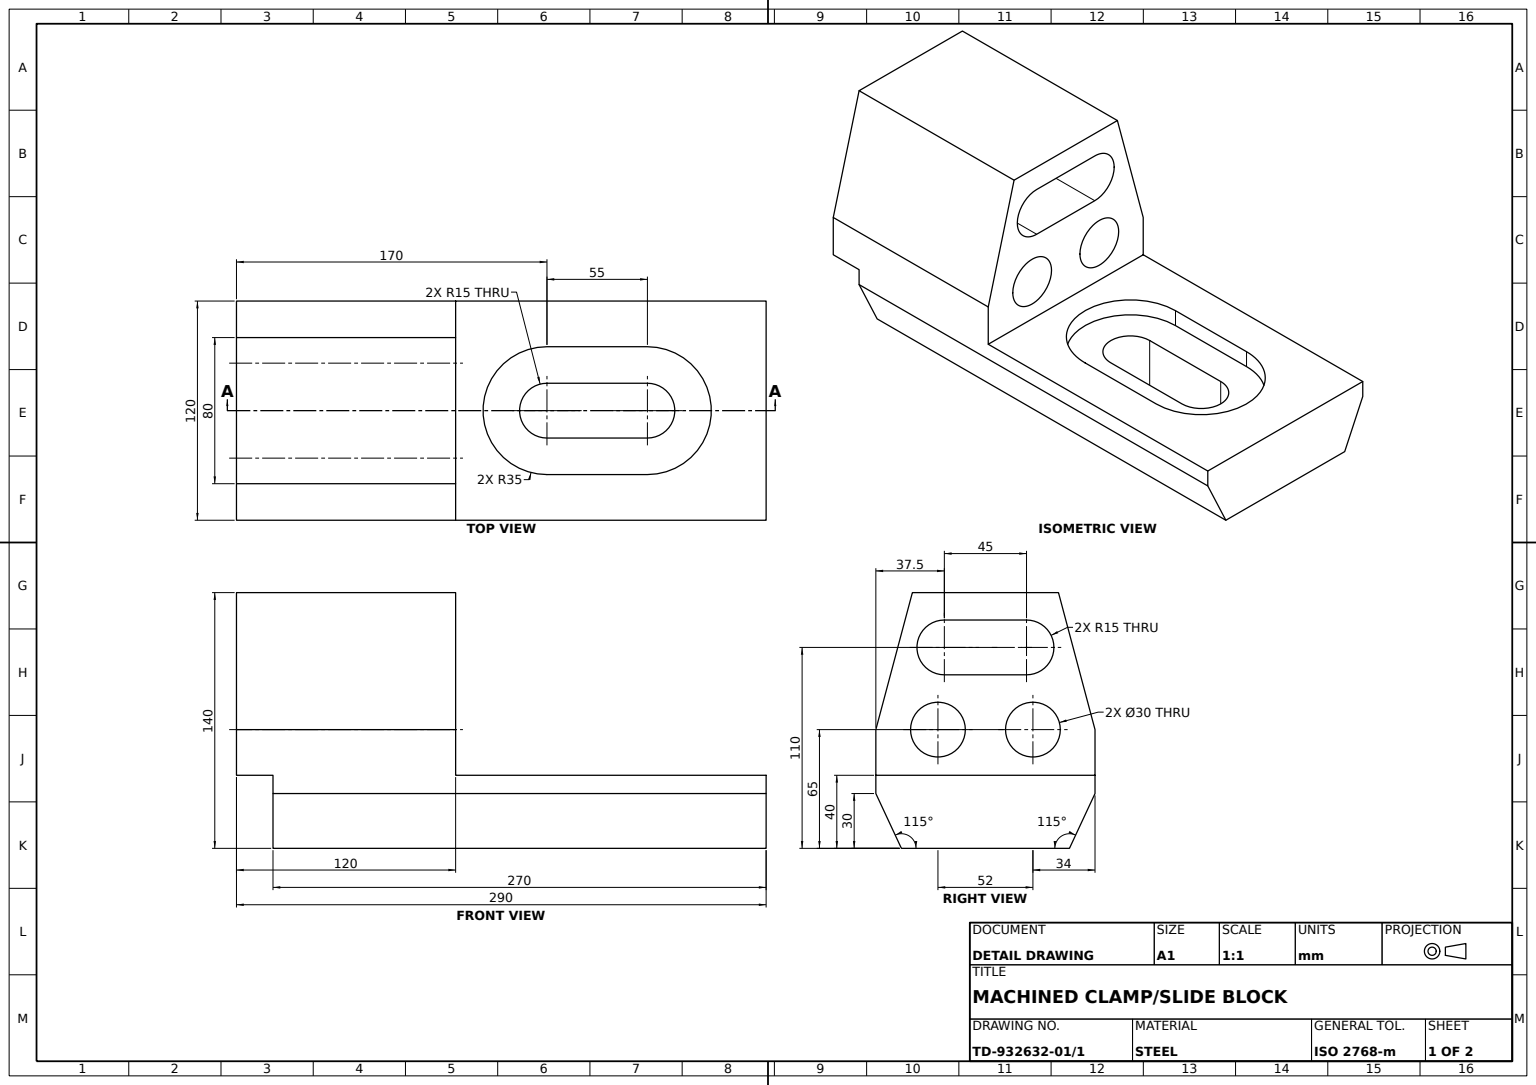
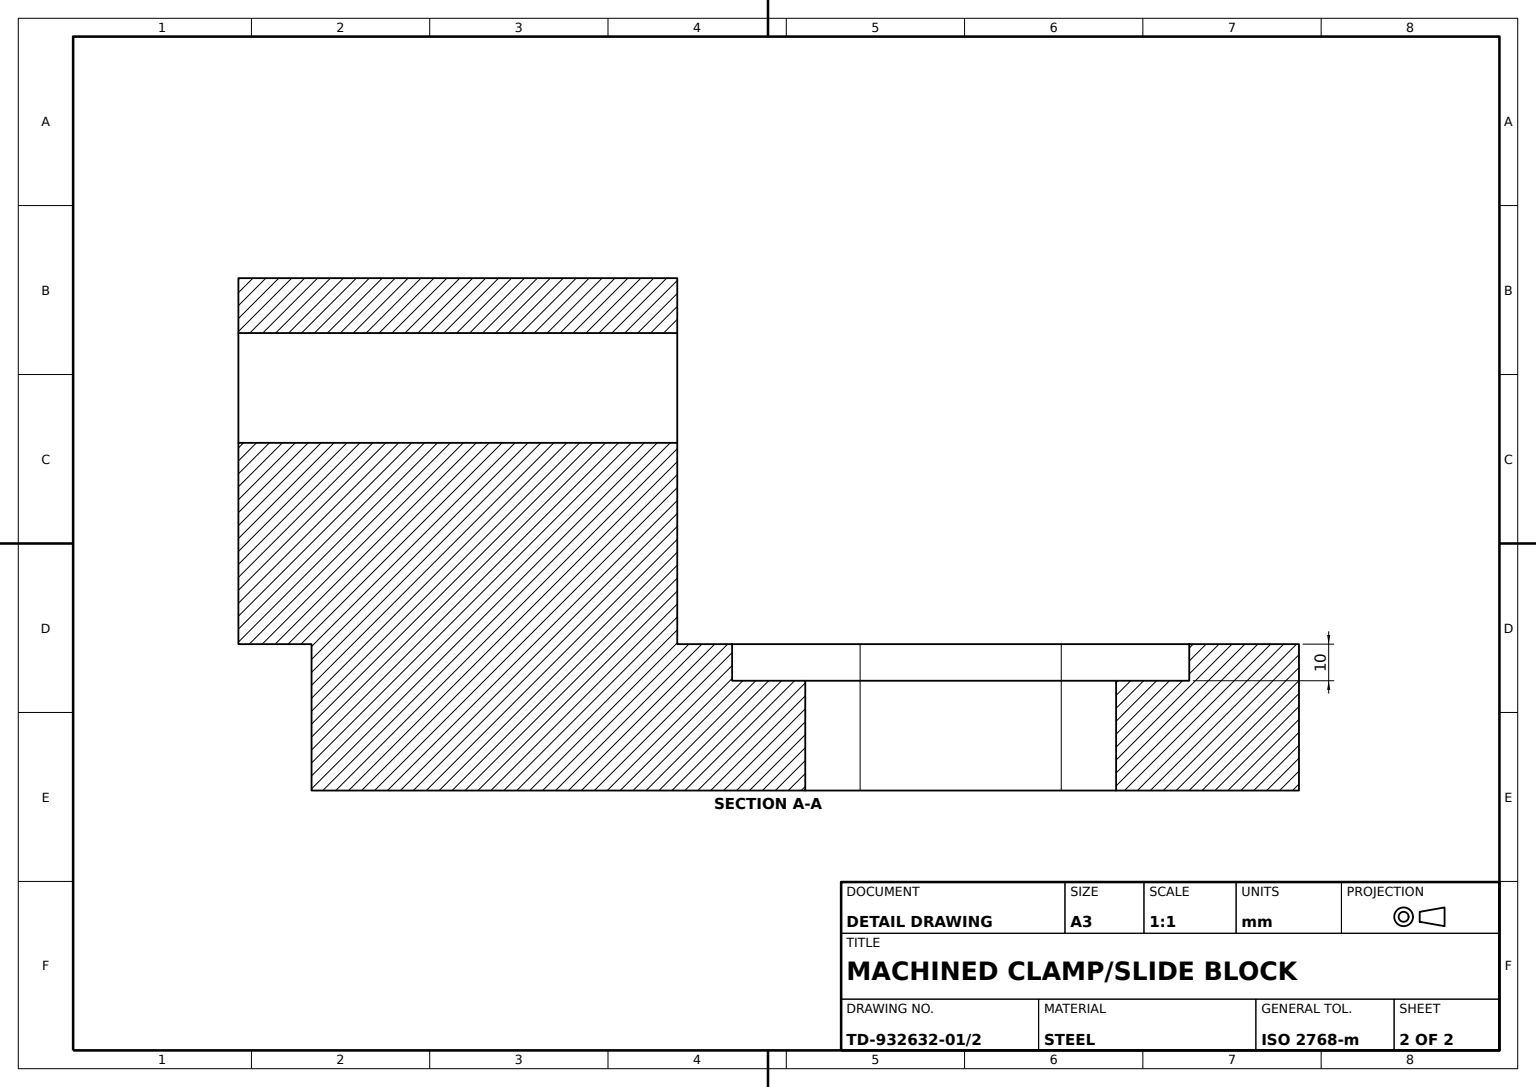
SolidWorks part; units mm, degrees
material "Plain Carbon Steel"
ref_plane "Front Plane" through (0, 0, 0) normal (0, 0, 1) x (1, 0, 0)
ref_plane "Top Plane" through (0, 0, 0) normal (0, 1, 0) x (1, 0, 0)
ref_plane "Right Plane" through (0, 0, 0) normal (1, 0, 0) x (0, 0, -1)
sketch "Wedge Rail Profile Sketch" plane through (0, 0, 0) normal (1, 0, 0) x (0, 0, -1)
  line L0 (-60, 0) -> (60, 0)
  line L1 (60, 0) -> (60, -10)
  line L2 (60, -10) -> (46.0108, -40)
  line L3 (46.0108, -40) -> (-46.0108, -40)
  line L4 (0, 0) -> (0, -51.1604) construction
  line L5 (-60, -10) -> (-46.0108, -40)
  line L6 (-60, 0) -> (-60, -10)
  point P8 (0, -40)
  dimension "D1" = 60
  dimension "D2" = 10
  dimension "D3" = 40
  dimension "D4" = 115
extrude "Wedge Base Rail" add sketch "Wedge Rail Profile Sketch" along normal mid plane 270
sketch "Upright Block Sketch" plane through (-135, 0, 0) normal (-1, 0, 0) x (0, 0, 1)
  line L0 (-60, 0) -> (-60, 25)
  line L1 (-60, 25) -> (-40, 100)
  line L2 (-40, 100) -> (40, 100)
  line L3 (40, 100) -> (60, 25)
  line L4 (60, 25) -> (60, 0)
  line L6 (-60, 0) -> (60, 0) construction
  line L7 (-60, 0) -> (60, 0)
  point P3 (0, 100)
  dimension "D1" = 80
  dimension "D2" = 100
  dimension "D3" = 25
extrude "Upright Block" add sketch "Upright Block Sketch" against normal blind 120 from offset 20
sketch "Block Slot and Holes Sketch" plane through (-35, 0, 0) normal (1, 0, 0) x (0, 0, -1)
  line L0 (60, 0) -> (-60, 0) construction
  line L1 (-22.5, 70) -> (22.5, 70) construction
  line L2 (-22.5, 85) -> (22.5, 85)
  line L3 (-22.5, 55) -> (22.5, 55)
  circle A0 centre (-26, 25) radius 15
  circle A1 centre (26, 25) radius 15
  arc A2 (-22.5, 85) -> (-22.5, 55) centre (-22.5, 70) ccw
  arc A3 (22.5, 55) -> (22.5, 85) centre (22.5, 70) ccw
  point P8 (0, 70)
  dimension "D1" = 30
  dimension "D6" = 15
  dimension "D2" = 25
  dimension "D3" = 52
  dimension "D4" = 26
  dimension "D5" = 45
  dimension "D7" = 70
extrude "Block Slot and Holes 2x" cut sketch "Block Slot and Holes Sketch" against normal blind 120
sketch "Slot Counterbore Sketch" plane through (0, 0, 0) normal (0, 1, 0) x (1, 0, 0)
  line L0 (15, 0) -> (70, 0) construction
  line L1 (15, 35) -> (70, 35)
  line L2 (15, -35) -> (70, -35)
  line L3 (135, 60) -> (135, -60) construction
  arc A0 (15, 35) -> (15, -35) centre (15, 0) ccw
  arc A1 (70, -35) -> (70, 35) centre (70, 0) ccw
  point P3 (42.5, 0)
  dimension "D1" = 70
  dimension "D2" = 65
  dimension "D3" = 120
extrude "Slot Counterbore Pocket" cut sketch "Slot Counterbore Sketch" against normal blind 10
sketch "Adjustment Slot Sketch" plane through (0, -10, 0) normal (0, 1, 0) x (1, 0, 0)
  line L0 (15, 0) -> (70, 0) construction
  line L1 (15, 15) -> (70, 15)
  line L2 (15, -15) -> (70, -15)
  arc A0 (15, 15) -> (15, -15) centre (15, 0) ccw
  arc A1 (70, -15) -> (70, 15) centre (70, 0) ccw
  arc A2 (15, 35) -> (15, -35) centre (15, 0) ccw construction
  arc A3 (70, -35) -> (70, 35) centre (70, 0) ccw construction
  point P3 (42.5, 0)
  dimension "D1" = 30
extrude "Adjustment Slot Through" cut sketch "Adjustment Slot Sketch" against normal through all
